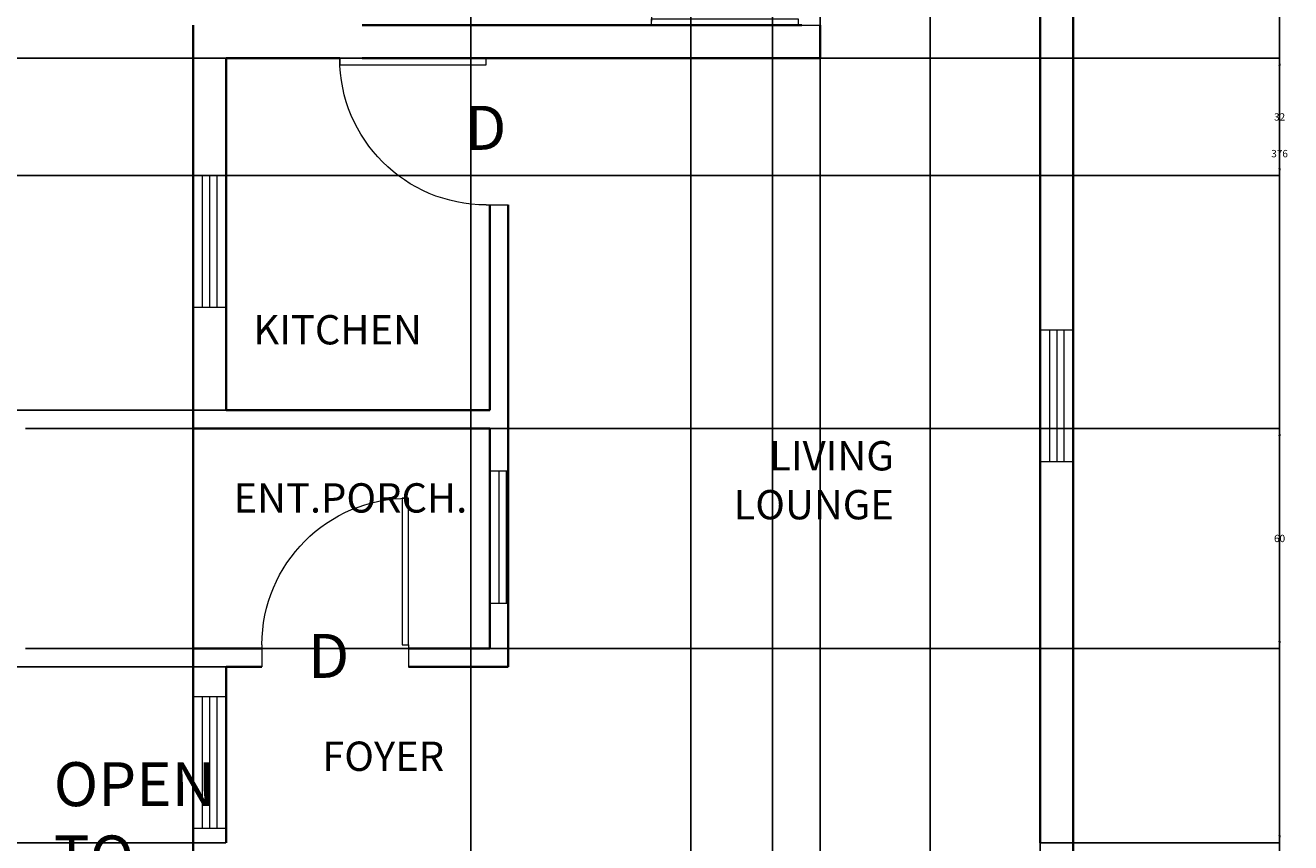
# Model space of a CAD drawing. Units: inches. Extents: x 190 to 836, y -241 to 999.
# Tile 8 of 9: x 491 to 836, y 566 to 789. Entities that reach past the tile are written whole.
import ezdxf

# ---------------------------------------------------------------- set-up
doc = ezdxf.new("R2010")
doc.units = ezdxf.units.IN
doc.header["$MEASUREMENT"] = 0
for name, color, linetype, lineweight in [('A-ANNO-DIMS', 2, 'Continuous', 18), ('A-ANNO-TEXT', 7, 'Continuous', 18), ('A-AREA-IDEN', 7, 'Continuous', 18), ('A-DOOR', 3, 'Continuous', 18), ('A-GLAZ', 4, 'Continuous', 18), ('A-WALL', 7, 'Continuous', 35)]:
    doc.layers.add(name, color=color, linetype=linetype, lineweight=lineweight)
doc.styles.get("Standard").update_dxf_attribs({"font": 'arial.ttf'})
doc.dimstyles.get("Standard").update_dxf_attribs({"dimtxt": 2, "dimasz": 2, "dimexe": 0.18, "dimexo": 0.0625, "dimgap": 0.09, "dimtad": 0, "dimtih": 1, "dimtoh": 1, "dimdec": 0, "dimzin": 0, "dimdsep": 46, "dimlunit": 3, "dimtxsty": 'Standard', "dimcen": 0.09, "dimadec": 0, "dimazin": 0, "dimtfac": 1, "dimtdec": 0, "dimtofl": 0, "dimtmove": 0, "dimatfit": 3, "dimfxl": 1, "dimtolj": 1, "dimtzin": 0, "dimarcsym": 0})

# ---------------------------------------------------------------- blocks, each defined once
blk = doc.blocks.new('*U2')
for p, q in [((0, 0), (0, 6)), ((40, 0), (40, 6))]:
    blk.add_line(p, q)
blk.add_lwpolyline([(0, 0), (0, -40), (1.75, -40), (1.75, 0)], close=True)
blk.add_arc((0, 0), 40, 270, 360)
blk = doc.blocks.new('*U4')
for p, q in [((-40, 0), (-40, 6)), ((0, 0), (0, 6))]:
    blk.add_line(p, q)
blk.add_lwpolyline([(0, 0), (0, -40), (-1.75, -40), (-1.75, 0)], close=True)
blk.add_arc((0, 0), 40, 180, 270)
blk = doc.blocks.new('*U5')
for p, q in [((0, 0), (0, -6)), ((40, 0), (40, -6))]:
    blk.add_line(p, q)
blk.add_lwpolyline([(0, 0), (0, 40), (1.75, 40), (1.75, 0)], close=True)
blk.add_arc((0, 0), 40, 0, 90)
blk = doc.blocks.new('WIN-36IN-9IN-3LINE')
for p, q in [((2.5, 36), (2.5, 0)), ((4.5, 36), (4.5, 0)), ((6.5, 36), (6.5, 0))]:
    blk.add_line(p, q)
blk.add_lwpolyline([(0, 0), (9, 0), (9, 36), (0, 36)], close=True)
blk = doc.blocks.new('WIN-36IN-5IN-PARTITION')
for p, q in [((5, 36), (0, 36)), ((0.5, 36), (0.5, 0)), ((2.5, 36), (2.5, 0)), ((5, 0), (5, 36)), ((0, 0), (5, 0))]:
    blk.add_line(p, q)
blk = doc.blocks.new('*D18')
at = {"layer": 'A-ANNO-DIMS', "color": 0, "lineweight": -2, "transparency": 16777216}
for p, q in [((776.5, 941.53), (832.94, 941.53)), ((832.76, 939.53), (832.76, 403.14)), ((832.76, -135.47), (832.76, 400.92)), ((776.5, -137.47), (832.94, -137.47))]:
    blk.add_line(p, q, dxfattribs=at)
at = {"layer": 'A-ANNO-DIMS', "color": 0, "transparency": 16777216}
for points in [[(832.43, 939.53), (833.1, 939.53), (832.76, 941.53)], [(832.43, -135.47), (833.1, -135.47), (832.76, -137.47)]]:
    blk.add_solid(points, dxfattribs=at)
at = {"layer": 'Defpoints', "color": 0, "transparency": 16777216}
for p in [(776.44, 941.53), (832.76, 941.53), (776.44, -137.47)]:
    blk.add_point(p, dxfattribs=at)
at = {"layer": 'A-ANNO-DIMS', "color": 0, "transparency": 16777216, "insert": (832.76, 402.03), "char_height": 2, "attachment_point": 5}
blk.add_mtext('\\A1;1079', dxfattribs=at)
blk = doc.blocks.new('*D21')
at = {"layer": 'A-ANNO-DIMS', "color": 0, "lineweight": -2, "transparency": 16777216}
for p, q in [((776.5, 941.53), (832.94, 941.53)), ((832.76, 939.53), (832.76, 754.64)), ((832.76, 567.53), (832.76, 752.42)), ((767.5, 565.53), (832.94, 565.53))]:
    blk.add_line(p, q, dxfattribs=at)
at = {"layer": 'A-ANNO-DIMS', "color": 0, "transparency": 16777216}
for points in [[(832.43, 939.53), (833.1, 939.53), (832.76, 941.53)], [(832.43, 567.53), (833.1, 567.53), (832.76, 565.53)]]:
    blk.add_solid(points, dxfattribs=at)
at = {"layer": 'Defpoints', "color": 0, "transparency": 16777216}
for p in [(776.44, 941.53), (832.76, 941.53), (767.44, 565.53)]:
    blk.add_point(p, dxfattribs=at)
at = {"layer": 'A-ANNO-DIMS', "color": 0, "transparency": 16777216, "insert": (832.76, 753.53), "char_height": 2, "attachment_point": 5}
blk.add_mtext('\\A1;376', dxfattribs=at)
blk = doc.blocks.new('*D27')
at = {"layer": 'A-ANNO-DIMS', "color": 0, "lineweight": -2, "transparency": 16777216}
for p, q in [((545.27, 779.53), (193.96, 779.53)), ((194.14, 777.53), (194.14, 732.64)), ((194.14, 685.53), (194.14, 730.42)), ((545.27, 683.53), (193.96, 683.53))]:
    blk.add_line(p, q, dxfattribs=at)
at = {"layer": 'A-ANNO-DIMS', "color": 0, "transparency": 16777216}
for points in [[(193.8, 777.53), (194.47, 777.53), (194.14, 779.53)], [(193.8, 685.53), (194.47, 685.53), (194.14, 683.53)]]:
    blk.add_solid(points, dxfattribs=at)
at = {"layer": 'Defpoints', "color": 0, "transparency": 16777216}
for p in [(194.14, 779.53), (545.33, 779.53), (545.33, 683.53)]:
    blk.add_point(p, dxfattribs=at)
at = {"layer": 'A-ANNO-DIMS', "color": 0, "transparency": 16777216, "insert": (194.14, 731.53), "char_height": 2, "attachment_point": 5}
blk.add_mtext('\\A1;96', dxfattribs=at)
blk = doc.blocks.new('*D28')
at = {"layer": 'A-ANNO-DIMS', "color": 0, "lineweight": -2, "transparency": 16777216}
for p, q in [((490.62, 678.53), (832.94, 678.53)), ((832.76, 676.53), (832.76, 649.64)), ((832.76, 620.53), (832.76, 647.42)), ((490.62, 618.53), (832.94, 618.53))]:
    blk.add_line(p, q, dxfattribs=at)
at = {"layer": 'A-ANNO-DIMS', "color": 0, "transparency": 16777216}
for points in [[(832.43, 676.53), (833.1, 676.53), (832.76, 678.53)], [(832.43, 620.53), (833.1, 620.53), (832.76, 618.53)]]:
    blk.add_solid(points, dxfattribs=at)
at = {"layer": 'Defpoints', "color": 0, "transparency": 16777216}
for p in [(490.55, 678.53), (832.76, 678.53), (490.55, 618.53)]:
    blk.add_point(p, dxfattribs=at)
at = {"layer": 'A-ANNO-DIMS', "color": 0, "transparency": 16777216, "insert": (832.76, 648.53), "char_height": 2, "attachment_point": 5}
blk.add_mtext('\\A1;60', dxfattribs=at)
blk = doc.blocks.new('*D30')
at = {"layer": 'A-ANNO-DIMS', "color": 0, "lineweight": -2, "transparency": 16777216}
for p, q in [((545.27, 613.53), (193.96, 613.53)), ((194.14, 611.53), (194.14, 590.64)), ((194.14, 567.53), (194.14, 588.42)), ((545.27, 565.53), (193.96, 565.53))]:
    blk.add_line(p, q, dxfattribs=at)
at = {"layer": 'A-ANNO-DIMS', "color": 0, "transparency": 16777216}
for points in [[(193.8, 611.53), (194.47, 611.53), (194.14, 613.53)], [(193.8, 567.53), (194.47, 567.53), (194.14, 565.53)]]:
    blk.add_solid(points, dxfattribs=at)
at = {"layer": 'Defpoints', "color": 0, "transparency": 16777216}
for p in [(194.14, 613.53), (545.33, 613.53), (545.33, 565.53)]:
    blk.add_point(p, dxfattribs=at)
at = {"layer": 'A-ANNO-DIMS', "color": 0, "transparency": 16777216, "insert": (194.14, 589.53), "char_height": 2, "attachment_point": 5}
blk.add_mtext('\\A1;48', dxfattribs=at)
blk = doc.blocks.new('*D31')
at = {"layer": 'A-ANNO-DIMS', "color": 0, "lineweight": -2, "transparency": 16777216}
for p, q in [((707.44, 855.47), (707.44, -239.95)), ((737.44, 855.47), (737.44, -239.95)), ((709.44, -239.77), (720.92, -239.77)), ((735.44, -239.77), (723.96, -239.77))]:
    blk.add_line(p, q, dxfattribs=at)
at = {"layer": 'A-ANNO-DIMS', "color": 0, "transparency": 16777216}
for points in [[(709.44, -239.44), (709.44, -240.11), (707.44, -239.77)], [(735.44, -239.44), (735.44, -240.11), (737.44, -239.77)]]:
    blk.add_solid(points, dxfattribs=at)
at = {"layer": 'Defpoints', "color": 0, "transparency": 16777216}
for p in [(707.44, 855.53), (737.44, 855.53), (707.44, -239.77)]:
    blk.add_point(p, dxfattribs=at)
at = {"layer": 'A-ANNO-DIMS', "color": 0, "transparency": 16777216, "insert": (722.44, -239.77), "char_height": 2, "attachment_point": 5}
blk.add_mtext('\\A1;30', dxfattribs=at)
blk = doc.blocks.new('*D43')
at = {"layer": 'A-ANNO-DIMS', "color": 0, "lineweight": -2, "transparency": 16777216}
for p, q in [((694.44, -128.41), (694.44, 998.02)), ((696.44, 997.84), (729.43, 997.84)), ((765.44, 997.84), (732.45, 997.84)), ((767.44, -128.41), (767.44, 998.02))]:
    blk.add_line(p, q, dxfattribs=at)
at = {"layer": 'A-ANNO-DIMS', "color": 0, "transparency": 16777216}
for points in [[(696.44, 998.17), (696.44, 997.5), (694.44, 997.84)], [(765.44, 998.17), (765.44, 997.5), (767.44, 997.84)]]:
    blk.add_solid(points, dxfattribs=at)
at = {"layer": 'Defpoints', "color": 0, "transparency": 16777216}
for p in [(767.44, 997.84), (694.44, -128.47), (767.44, -128.47)]:
    blk.add_point(p, dxfattribs=at)
at = {"layer": 'A-ANNO-DIMS', "color": 0, "transparency": 16777216, "insert": (730.94, 997.84), "char_height": 2, "attachment_point": 5}
blk.add_mtext('\\A1;73', dxfattribs=at)
blk = doc.blocks.new('*D45')
at = {"layer": 'A-ANNO-DIMS', "color": 0, "lineweight": -2, "transparency": 16777216}
for p, q in [((612.1, 115.59), (612.1, 998.02)), ((614.1, 997.84), (640.58, 997.84)), ((670.1, 997.84), (643.62, 997.84)), ((672.1, 115.59), (672.1, 998.02))]:
    blk.add_line(p, q, dxfattribs=at)
at = {"layer": 'A-ANNO-DIMS', "color": 0, "transparency": 16777216}
for points in [[(614.1, 998.17), (614.1, 997.5), (612.1, 997.84)], [(670.1, 998.17), (670.1, 997.5), (672.1, 997.84)]]:
    blk.add_solid(points, dxfattribs=at)
at = {"layer": 'Defpoints', "color": 0, "transparency": 16777216}
for p in [(672.1, 997.84), (612.1, 115.53), (672.1, 115.53)]:
    blk.add_point(p, dxfattribs=at)
at = {"layer": 'A-ANNO-DIMS', "color": 0, "transparency": 16777216, "insert": (642.1, 997.84), "char_height": 2, "attachment_point": 5}
blk.add_mtext('\\A1;60', dxfattribs=at)
blk = doc.blocks.new('*D46')
at = {"layer": 'A-ANNO-DIMS', "color": 0, "lineweight": -2, "transparency": 16777216}
for p, q in [((707.44, 120.59), (707.44, 998.02)), ((709.44, 997.84), (735.92, 997.84)), ((765.44, 997.84), (738.97, 997.84)), ((767.44, 120.59), (767.44, 998.02))]:
    blk.add_line(p, q, dxfattribs=at)
at = {"layer": 'A-ANNO-DIMS', "color": 0, "transparency": 16777216}
for points in [[(709.44, 998.17), (709.44, 997.5), (707.44, 997.84)], [(765.44, 998.17), (765.44, 997.5), (767.44, 997.84)]]:
    blk.add_solid(points, dxfattribs=at)
at = {"layer": 'Defpoints', "color": 0, "transparency": 16777216}
for p in [(767.44, 997.84), (707.44, 120.53), (767.44, 120.53)]:
    blk.add_point(p, dxfattribs=at)
at = {"layer": 'A-ANNO-DIMS', "color": 0, "transparency": 16777216, "insert": (737.44, 997.84), "char_height": 2, "attachment_point": 5}
blk.add_mtext('\\A1;60', dxfattribs=at)
blk = doc.blocks.new('*D53')
at = {"layer": 'A-ANNO-DIMS', "color": 0, "lineweight": -2, "transparency": 16777216}
for p, q in [((481.62, 779.53), (832.94, 779.53)), ((832.76, 777.53), (832.76, 764.64)), ((832.76, 749.53), (832.76, 762.42)), ((481.6, 747.53), (832.94, 747.53))]:
    blk.add_line(p, q, dxfattribs=at)
at = {"layer": 'A-ANNO-DIMS', "color": 0, "transparency": 16777216}
for points in [[(832.43, 777.53), (833.1, 777.53), (832.76, 779.53)], [(832.43, 749.53), (833.1, 749.53), (832.76, 747.53)]]:
    blk.add_solid(points, dxfattribs=at)
at = {"layer": 'Defpoints', "color": 0, "transparency": 16777216}
for p in [(481.55, 779.53), (832.76, 779.53), (481.54, 747.53)]:
    blk.add_point(p, dxfattribs=at)
at = {"layer": 'A-ANNO-DIMS', "color": 0, "transparency": 16777216, "insert": (832.76, 763.53), "char_height": 2, "attachment_point": 5}
blk.add_mtext('\\A1;32', dxfattribs=at)

msp = doc.modelspace()

# ---------------------------------------------------------------- linework, layer by layer
at = {"layer": 'A-WALL'}
for p, q in [((776.4421, 941.5313), (776.4421, 556.5313)), ((767.4421, 855.5313), (767.4421, 565.5313)), ((536.3307, 788.5313), (536.3307, 732.9119)), ((702.4421, 788.5313), (582.4421, 788.5313)), ((707.4421, 779.5313), (707.4421, 788.5313)), ((536.3307, 556.5313), (536.3307, 779.5313)), ((576.3307, 779.5313), (545.3307, 779.5313)), ((545.3307, 683.5313), (545.3307, 779.5313)), ((707.4421, 779.5313), (582.4421, 779.5313)), ((617.3307, 683.5313), (617.3307, 739.5313)), ((622.3307, 613.5313), (622.3307, 739.5313)), ((617.3307, 683.5313), (545.3307, 683.5313)), ((617.3307, 678.5313), (536.3307, 678.5313)), ((617.3307, 618.5313), (617.3307, 678.5313)), ((555.1115, 618.5313), (536.3307, 618.5313)), ((598.7702, 618.5313), (595.1115, 618.5313)), ((617.3307, 618.5313), (598.7702, 618.5313)), ((555.1115, 613.5313), (545.3307, 613.5313)), ((545.3307, 565.5313), (545.3307, 613.5313)), ((622.3307, 613.5313), (595.1115, 613.5313))]:
    msp.add_line(p, q, dxfattribs=at)

# ---------------------------------------------------------------- block references
at = {"layer": 'A-DOOR', "xscale": -1}
for name, p, rotation in [('*U2', (701.4421, 788.5313), 269.9999999999999), ('*U4', (616.3307, 779.5313), 269.9999999999999), ('*U5', (595.1115, 619.5313), 360)]:
    msp.add_blockref(name, p, dxfattribs=dict(at, rotation=rotation))
at = {"layer": 'A-GLAZ', "extrusion": (0, 0, -1), "zscale": -1}
for p in [(-545.3421, 711.532), (-776.4423, 669.4424), (-545.3309, 569.3993)]:
    msp.add_blockref('WIN-36IN-9IN-3LINE', p, dxfattribs=at)
at = {"layer": 'A-GLAZ', "rotation": 180}
msp.add_blockref('WIN-36IN-5IN-PARTITION', (622.3303, 666.9), dxfattribs=at)

# ---------------------------------------------------------------- texts
at = {"layer": 'A-ANNO-TEXT', "char_height": 12, "attachment_point": 3}
for insert in [(621.7996, 766.5566), (578.9435, 622.4981)]:
    msp.add_mtext_dynamic_manual_height_columns('D', width=8.765037, gutter_width=1, heights=[0], dxfattribs=dict(at, insert=insert))
at = {"layer": 'A-AREA-IDEN'}
for s, width, insert, char_height, attachment_point in [('KITCHEN', 33.040256, (598.7825, 709.4705), 8, 3), ('LIVING LOUNGE ', 33.040256, (727.5247, 675.086), 8, 3), ('ENT.PORCH.', 33.040256, (611.1309, 663.5955), 8, 3), ('FOYER', 33.040256, (604.8346, 593.1169), 8, 3), ('OPEN TO SKY', 38.023659, (498.3071, 587.4984), 12, 1)]:
    msp.add_mtext_dynamic_manual_height_columns(s, width=width, gutter_width=1, heights=[0], dxfattribs=dict(at, insert=insert, char_height=char_height, attachment_point=attachment_point))

# ---------------------------------------------------------------- dimensions: what is measured, and where the dimension line sits
at = {"layer": 'A-ANNO-DIMS'}
for base, p1, p2, picture, middle in [((672.0998, 997.8363), (612.0998, 115.5313), (672.0998, 115.5313), '*D45', (642.0998, 997.8363)), ((767.4421, 997.8363), (694.4376, -128.4687), (767.4421, -128.4687), '*D43', (730.9399, 997.8363)), ((767.4421, 997.8363), (707.4421, 120.5313), (767.4421, 120.5313), '*D46', (737.4421, 997.8363)), ((707.4421, -239.7737), (737.4421, 855.5313), (707.4421, 855.5313), '*D31', (722.4421, -239.7737))]:
    dim = msp.add_linear_dim(base=base, p1=p1, p2=p2, dimstyle='Standard', override={"dimdec": 0, "dimlfac": 1, "dimrnd": 0, "dimzin": 0, "dimdsep": 46, "dimlunit": 2}, dxfattribs=at)
    dim.commit()
    dim.dimension.update_dxf_attribs({"geometry": picture, "text_midpoint": middle})
for base, p1, p2, picture, middle in [((832.7634, 941.5313), (767.4421, 565.5313), (776.4421, 941.5313), '*D21', (832.7634, 753.5313)), ((832.7634, 941.5313), (776.4421, -137.4687), (776.4421, 941.5313), '*D18', (832.7634, 402.0313)), ((194.1371, 779.5313), (545.3307, 683.5313), (545.3307, 779.5313), '*D27', (194.1371, 731.5313)), ((832.7634, 779.5313), (481.5423, 747.5319), (481.5536, 779.5313), '*D53', (832.7634, 763.5316)), ((832.7634, 678.5313), (490.5536, 618.5313), (490.5536, 678.5313), '*D28', (832.7634, 648.5313)), ((194.1371, 613.5313), (545.3307, 565.5313), (545.3307, 613.5313), '*D30', (194.1371, 589.5313))]:
    dim = msp.add_linear_dim(base=base, p1=p1, p2=p2, angle=90, dimstyle='Standard', override={"dimdec": 0, "dimlfac": 1, "dimrnd": 0, "dimzin": 0, "dimdsep": 46, "dimlunit": 2}, dxfattribs=at)
    dim.commit()
    dim.dimension.update_dxf_attribs({"geometry": picture, "text_midpoint": middle})

doc.saveas('drawing.dxf')
